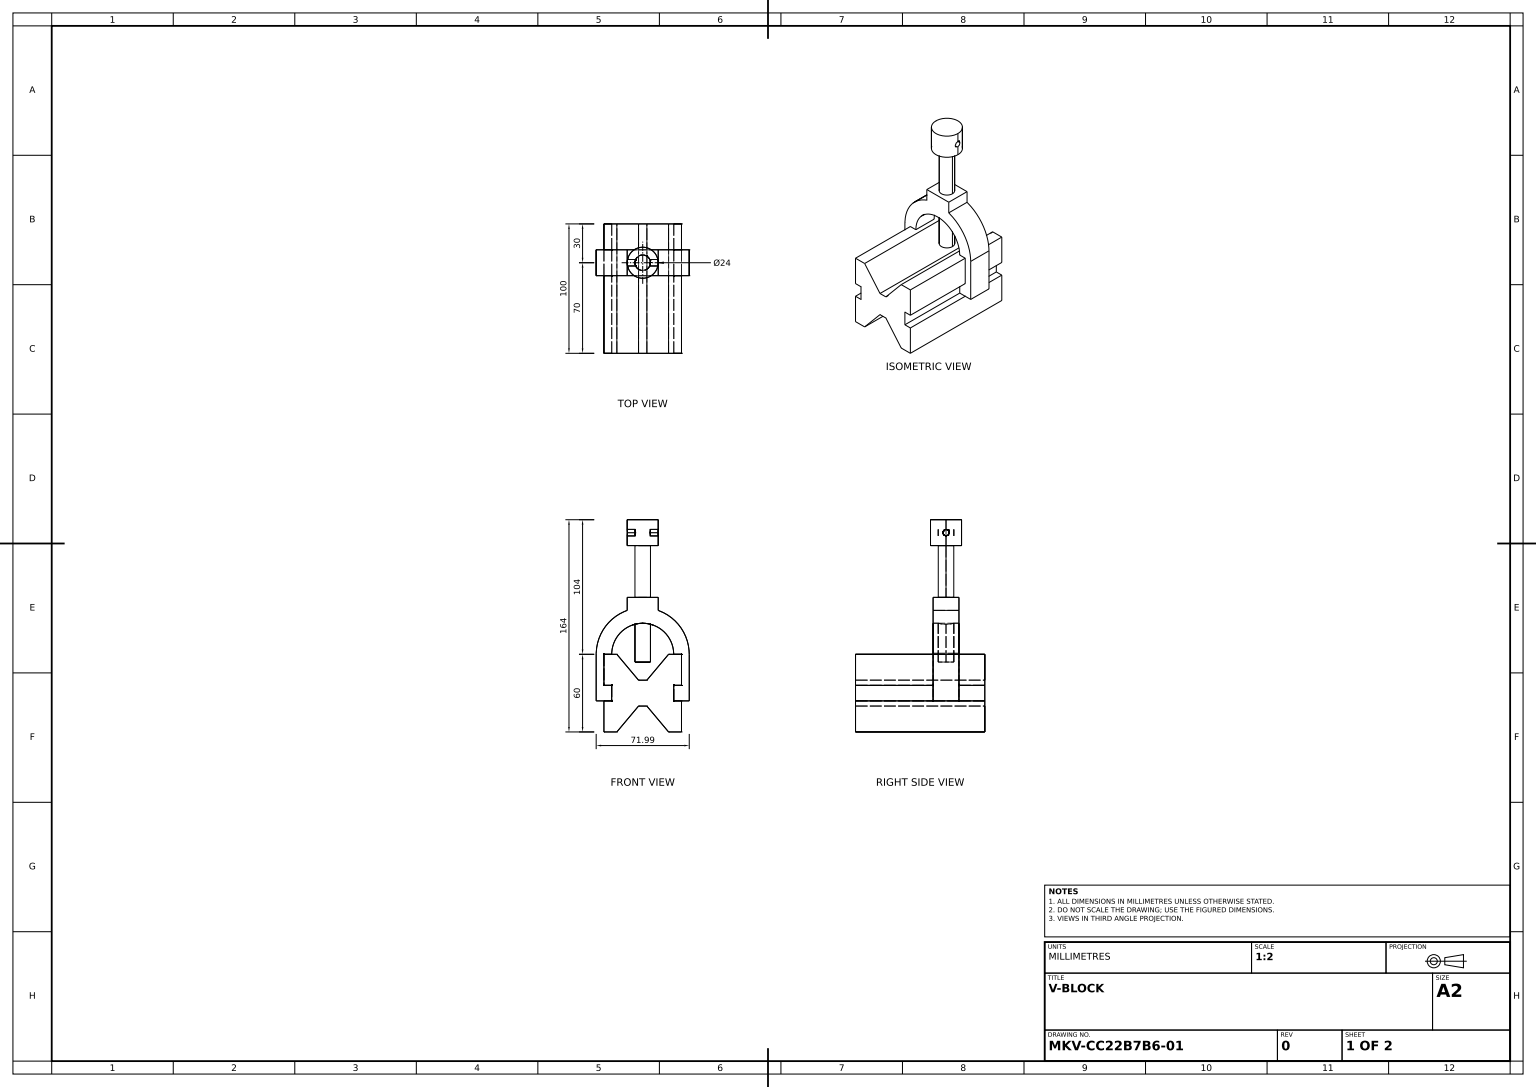
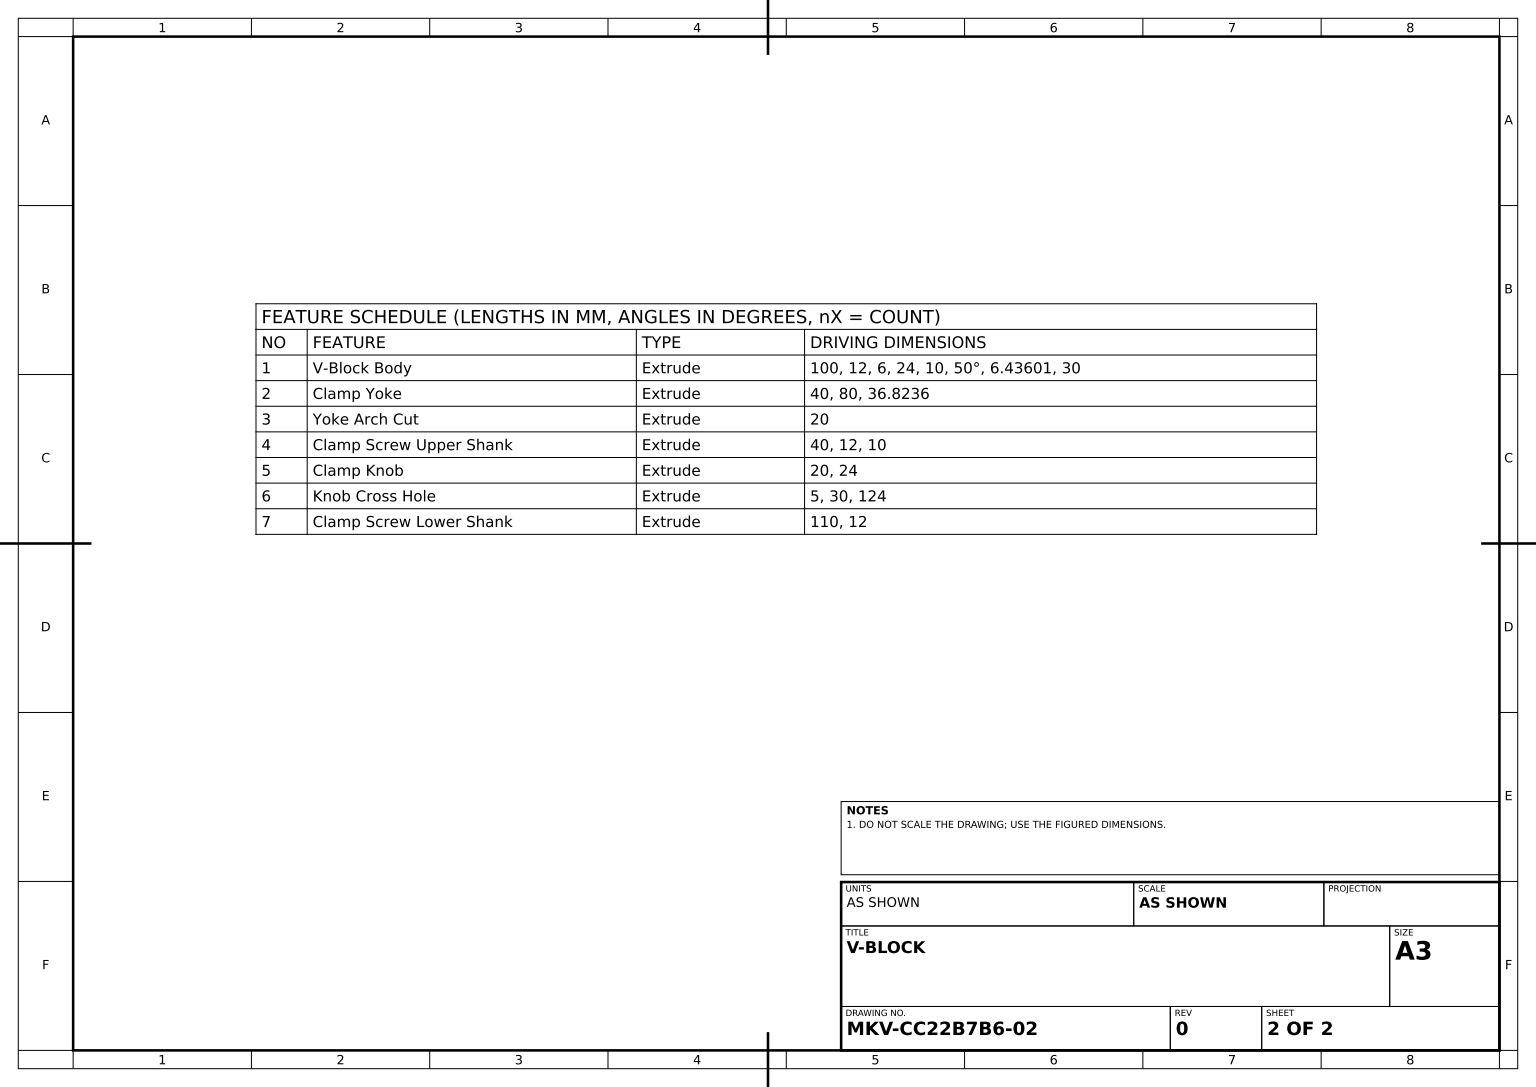
SolidWorks part; units mm, degrees
material "Plain Carbon Steel"
ref_plane "Front Plane" through (0, 0, 0) normal (0, 0, 1) x (1, 0, 0)
ref_plane "Top Plane" through (0, 0, 0) normal (0, 1, 0) x (1, 0, 0)
ref_plane "Right Plane" through (0, 0, 0) normal (1, 0, 0) x (0, 0, -1)
sketch "V-Block Profile Sketch" plane through (0, 0, 0) normal (0, 0, 1) x (1, 0, 0)
  line L0 (0, 0) -> (27.3391, 0) construction
  line L1 (-30, 30) -> (-20, 30)
  line L2 (-30, 30) -> (-30, 6)
  line L4 (30, 30) -> (30, 6)
  line L5 (-30, 30) -> (30, -30) construction
  line L6 (-30, -30) -> (30, 30) construction
  line L12 (0, 0) -> (0, 23.687) construction
  line L13 (-30, 6) -> (-24, 6)
  line L14 (-24, 6) -> (-24, -6)
  line L15 (-24, -6) -> (-30, -6)
  line L16 (-30, -6) -> (-30, -30)
  line L17 (24, -6) -> (30, -6)
  line L18 (24, 6) -> (24, -6)
  line L19 (30, 6) -> (24, 6)
  line L20 (30, -6) -> (30, -30)
  line L24 (20, 30) -> (30, 30)
  line L29 (20, 30) -> (3.218, 10)
  line L30 (-3.218, 10) -> (3.218, 10)
  line L31 (-20, -30) -> (-3.218, -10)
  line L32 (-3.218, -10) -> (3.218, -10)
  line L33 (20, -30) -> (3.218, -10)
  line L34 (0, 10) -> (-6.436, 10) construction
  line L35 (-20, 30) -> (-3.218, 10)
  line L38 (20, -30) -> (30, -30)
  line L39 (-30, -30) -> (-20, -30)
  point P0 (0, 0)
  dimension "D1" = 50
  dimension "D2" = 6.436
  dimension "D3" = 10
  dimension "D4" = 12
  dimension "D5" = 6
  dimension "D6" = 24
  dimension "D7" = 24
  dimension "D8" = 30
extrude "V-Block Body" add sketch "V-Block Profile Sketch" along normal blind 100
sketch "Clamp Yoke Sketch" plane through (0, 0, 0) normal (0, 0, -1) x (-1, 0, 0)
  line L0 (-12.5033, 74) -> (-36, 74) construction
  line L1 (-20, 30) -> (20, 30) construction
  line L2 (-24, -6) -> (-36, -6)
  line L3 (-36, -6) -> (-36, 30)
  line L4 (24, -6) -> (35.9906, -6)
  line L5 (0, 30) -> (0, 10) construction
  line L6 (-36, -6) -> (-36, 74) construction
  line L9 (12, 74) -> (-12, 74)
  line L11 (-12, 74) -> (-12, 63.9411)
  line L12 (35.9906, -6) -> (35.9906, 30.8236)
  line L13 (-24, -6) -> (-24, 6)
  line L14 (-24, 6) -> (-30, 6)
  line L15 (-30, 6) -> (-30, 30)
  line L16 (-30, 30) -> (-24, 30)
  line L20 (24, 30) -> (30, 30)
  line L21 (30, 30) -> (30, 6)
  line L22 (30, 6) -> (24, 6)
  line L23 (24, 6) -> (24, -6)
  line L24 (12, 74) -> (12, 63.9411)
  line L25 (0, 30) -> (0, 76.4819) construction
  arc A7 (24, 30) -> (-24, 30) centre (0, 30) ccw
  arc A8 (35.9906, 30.8236) -> (12, 63.9411) centre (0, 30) ccw
  arc A9 (-12, 63.9411) -> (-36, 30) centre (0, 30) ccw
  point P19 (0, 74)
  dimension "D2" = 80
  dimension "D4" = 36.8236
extrude "Clamp Yoke" add sketch "Clamp Yoke Sketch" against normal blind 40
sketch "Yoke Arch Cut Sketch" plane through (0, 0, 0) normal (0, 0, -1) x (-1, 0, 0)
  line L0 (-30, -6) -> (-36, -6)
  line L1 (-36, -6) -> (-36, 30)
  line L2 (-12, 63.9411) -> (-12, 74)
  line L3 (-12, 74) -> (-12, 63.9411) construction
  line L4 (-12, 74) -> (12, 74)
  line L5 (12, 74) -> (12, 63.9411)
  line L6 (35.9906, 30.8236) -> (35.9906, -6)
  line L7 (35.9906, -6) -> (30, -6)
  line L11 (-24, 30) -> (-20, 30) construction
  line L18 (0, 0) -> (0, 38.0472) construction
  line L22 (-30, -6) -> (-24, -6)
  line L23 (-24, -6) -> (-24, 6)
  line L24 (-24, 6) -> (-30, 6)
  line L25 (-30, 6) -> (-30, 30)
  line L26 (-30, 30) -> (-24, 30)
  line L27 (30, -6) -> (24, -6)
  line L28 (24, -6) -> (24, 6)
  line L29 (24, 6) -> (30, 6)
  line L30 (30, 6) -> (30, 30)
  line L31 (30, 30) -> (24, 30)
  arc A0 (-36, 30) -> (-12, 63.9411) centre (0, 30) cw
  arc A1 (12, 63.9411) -> (35.9906, 30.8236) centre (0, 30) cw
  arc A2 (24, 30) -> (-24, 30) centre (0, 30) ccw
extrude "Yoke Arch Cut" cut sketch "Yoke Arch Cut Sketch" against normal blind 20
sketch "Clamp Screw Upper Shank Sketch" plane through (0, 74, 0) normal (0, 1, 0) x (1, 0, 0)
  line L0 (12, -40) -> (12, -20) construction
  line L1 (-12, -20) -> (12, -20) construction
  circle A0 centre (0, -30) radius 6
  dimension "D1" = 12
  dimension "D2" = 12
  dimension "D3" = 10
extrude "Clamp Screw Upper Shank" add sketch "Clamp Screw Upper Shank Sketch" along normal blind 40
sketch "Clamp Knob Sketch" plane through (0, 114, 0) normal (0, 1, 0) x (1, 0, 0)
  circle A0 centre (0, -30) radius 12
  dimension "D1" = 24
extrude "Clamp Knob" add sketch "Clamp Knob Sketch" along normal blind 20
sketch "Knob Cross Hole Sketch" plane through (0, 0, 0) normal (1, 0, 0) x (0, 0, -1)
  circle A0 centre (-30, 124) radius 2.5
  dimension "D1" = 5
  dimension "D2" = 30
  dimension "D3" = 124
extrude "Knob Cross Hole" cut sketch "Knob Cross Hole Sketch" against normal through all both and the other way through all
sketch "Clamp Screw Lower Shank Sketch" plane through (0, 134, 0) normal (0, 1, 0) x (1, 0, 0)
  circle A0 centre (0, -30) radius 6
  dimension "D1" = 12
extrude "Clamp Screw Lower Shank" add sketch "Clamp Screw Lower Shank Sketch" against normal blind 110
